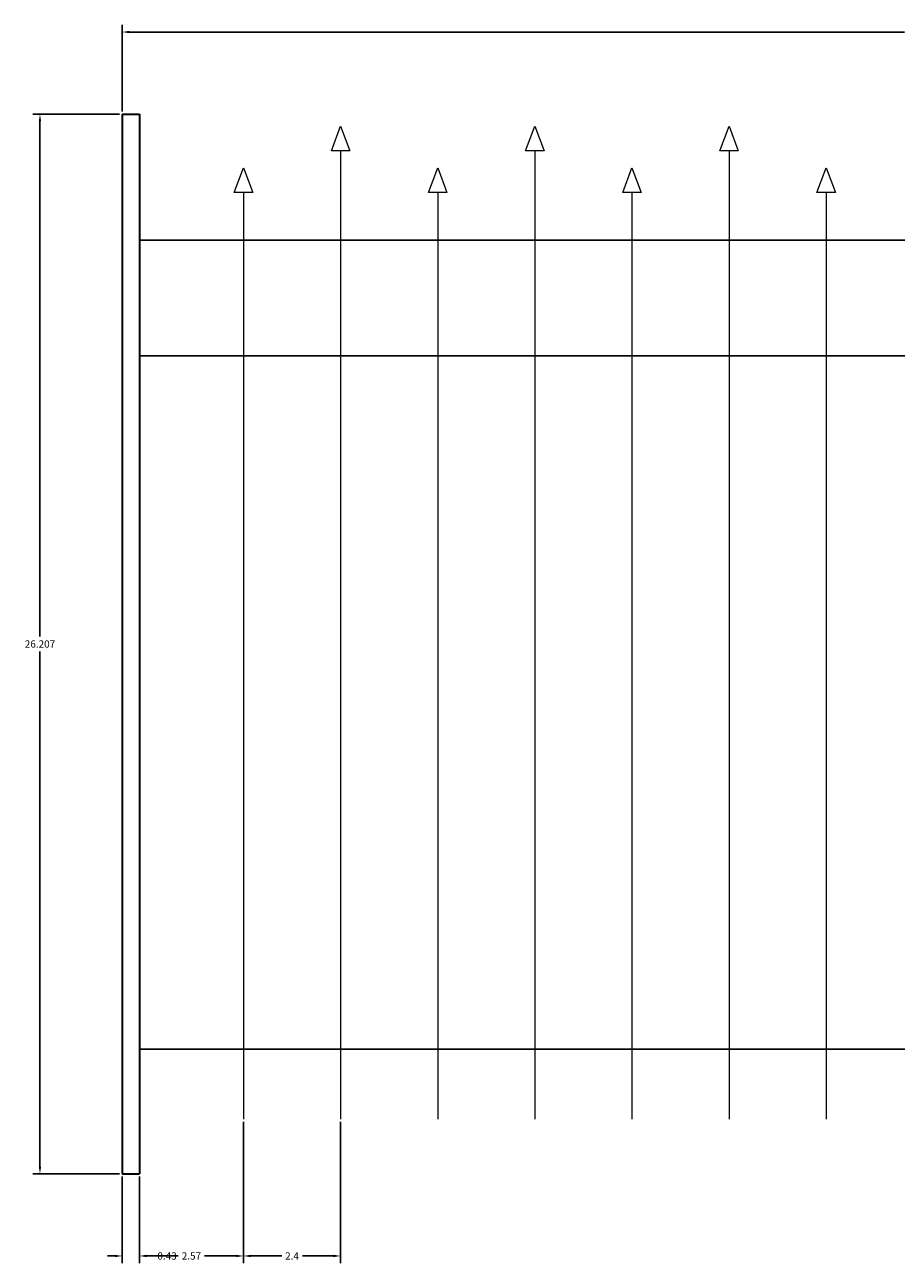
# Model space of a CAD drawing. Units: inches. Extents: x 756 to 915, y 488 to 695.
# Tile 17 of 25: x 768 to 789, y 664 to 694. Entities that reach past the tile are written whole.
import ezdxf

# ---------------------------------------------------------------- set-up
doc = ezdxf.new("R2010")
doc.units = ezdxf.units.IN
doc.header["$MEASUREMENT"] = 0
for name, color, linetype, lineweight in [('L-FENC-PCKT', 7, 'Continuous', 18), ('L-FENC-POST', 7, 'Continuous', 35), ('L-FENC-RAIL', 7, 'Continuous', 25), ('M-DIMS', 2, 'Continuous', 18)]:
    doc.layers.add(name, color=color, linetype=linetype, lineweight=lineweight)
doc.styles.get("Standard").update_dxf_attribs({"font": 'arial.ttf'})
doc.dimstyles.get("Standard").update_dxf_attribs({"dimtxt": 0.18, "dimasz": 0.18, "dimexe": 0.18, "dimexo": 0.0625, "dimgap": 0.09, "dimtad": 0, "dimtih": 1, "dimtoh": 1, "dimdec": 0, "dimzin": 0, "dimdsep": 46, "dimlunit": 3, "dimtxsty": 'Standard', "dimcen": 0.09, "dimadec": 0, "dimazin": 0, "dimtfac": 1, "dimtdec": 0, "dimtofl": 0, "dimtmove": 0, "dimatfit": 3, "dimfxl": 1, "dimtolj": 1, "dimtzin": 0, "dimarcsym": 0})

# ---------------------------------------------------------------- blocks, each defined once
blk = doc.blocks.new('PICKET-SPEAR-EXTENDED')
blk.add_line((0.228, 23.946), (0.228, 0))
blk.add_lwpolyline([(0.228, 23.946), (0, 23.946), (0.228, 24.558), (0.455, 23.946)], close=True)
blk = doc.blocks.new('FENCE-POST-LEFT')
for p, q in [((0, 26.207), (0, 0)), ((0, 26.207), (0.426, 26.207)), ((0.426, 26.207), (0.426, 0)), ((0.426, 26.207), (0.426, 0)), ((0, 0), (0.426, 0))]:
    blk.add_line(p, q)
blk = doc.blocks.new('PICKET-SPEAR-LOW')
blk.add_line((0.228, 22.916), (0.228, 0))
blk.add_lwpolyline([(0.228, 22.916), (0, 22.916), (0.228, 23.528), (0.455, 22.916)], close=True)
blk = doc.blocks.new('*D13')
at = {"layer": 'Defpoints', "color": 0, "transparency": 16777216}
for p in [(809.674, 693.983), (770.216, 691.953), (809.674, 691.953)]:
    blk.add_point(p, dxfattribs=at)
at = {"layer": 'M-DIMS', "color": 0, "lineweight": -2, "transparency": 16777216}
for p, q in [((770.216, 692.015), (770.216, 694.163)), ((809.674, 692.015), (809.674, 694.163)), ((770.396, 693.983), (789.551, 693.983)), ((809.494, 693.983), (790.338, 693.983))]:
    blk.add_line(p, q, dxfattribs=at)
at = {"layer": 'M-DIMS', "color": 0, "transparency": 16777216}
for points in [[(770.396, 694.013), (770.396, 693.953), (770.216, 693.983)], [(809.494, 694.013), (809.494, 693.953), (809.674, 693.983)]]:
    blk.add_solid(points, dxfattribs=at)
at = {"layer": 'M-DIMS', "color": 0, "transparency": 16777216, "insert": (789.945, 693.983), "char_height": 0.18, "attachment_point": 5}
blk.add_mtext('\\A1;39.46', dxfattribs=at)
blk = doc.blocks.new('*D14')
at = {"layer": 'Defpoints', "color": 0, "transparency": 16777216}
for p in [(768.186, 691.953), (770.216, 691.953), (770.216, 665.746)]:
    blk.add_point(p, dxfattribs=at)
at = {"layer": 'M-DIMS', "color": 0, "lineweight": -2, "transparency": 16777216}
for p, q in [((770.153, 691.953), (768.006, 691.953)), ((768.186, 691.773), (768.186, 679.031)), ((768.186, 665.926), (768.186, 678.668)), ((770.153, 665.746), (768.006, 665.746))]:
    blk.add_line(p, q, dxfattribs=at)
at = {"layer": 'M-DIMS', "color": 0, "transparency": 16777216}
for points in [[(768.156, 691.773), (768.216, 691.773), (768.186, 691.953)], [(768.156, 665.926), (768.216, 665.926), (768.186, 665.746)]]:
    blk.add_solid(points, dxfattribs=at)
at = {"layer": 'M-DIMS', "color": 0, "transparency": 16777216, "insert": (768.186, 678.849), "char_height": 0.18, "attachment_point": 5}
blk.add_mtext('\\A1;26.207', dxfattribs=at)
blk = doc.blocks.new('*D15')
at = {"layer": 'Defpoints', "color": 0, "transparency": 16777216}
for p in [(773.215, 667.096), (775.615, 667.096), (775.615, 663.716)]:
    blk.add_point(p, dxfattribs=at)
at = {"layer": 'M-DIMS', "color": 0, "lineweight": -2, "transparency": 16777216}
for p, q in [((773.215, 667.033), (773.215, 663.536)), ((775.615, 667.033), (775.615, 663.536)), ((773.395, 663.716), (774.16, 663.716)), ((775.435, 663.716), (774.67, 663.716))]:
    blk.add_line(p, q, dxfattribs=at)
at = {"layer": 'M-DIMS', "color": 0, "transparency": 16777216}
for points in [[(773.395, 663.746), (773.395, 663.686), (773.215, 663.716)], [(775.435, 663.746), (775.435, 663.686), (775.615, 663.716)]]:
    blk.add_solid(points, dxfattribs=at)
at = {"layer": 'M-DIMS', "color": 0, "transparency": 16777216, "insert": (774.415, 663.716), "char_height": 0.18, "attachment_point": 5}
blk.add_mtext('\\A1;2.4', dxfattribs=at)
blk = doc.blocks.new('*D16')
at = {"layer": 'Defpoints', "color": 0, "transparency": 16777216}
for p in [(773.215, 667.096), (770.642, 665.746), (773.215, 663.716)]:
    blk.add_point(p, dxfattribs=at)
at = {"layer": 'M-DIMS', "color": 0, "lineweight": -2, "transparency": 16777216}
for p, q in [((773.215, 667.033), (773.215, 663.536)), ((770.642, 665.684), (770.642, 663.536)), ((770.822, 663.716), (771.603, 663.716)), ((773.035, 663.716), (772.254, 663.716))]:
    blk.add_line(p, q, dxfattribs=at)
at = {"layer": 'M-DIMS', "color": 0, "transparency": 16777216}
for points in [[(770.822, 663.746), (770.822, 663.686), (770.642, 663.716)], [(773.035, 663.746), (773.035, 663.686), (773.215, 663.716)]]:
    blk.add_solid(points, dxfattribs=at)
at = {"layer": 'M-DIMS', "color": 0, "transparency": 16777216, "insert": (771.929, 663.716), "char_height": 0.18, "attachment_point": 5}
blk.add_mtext('\\A1;2.57', dxfattribs=at)
blk = doc.blocks.new('*D18')
at = {"layer": 'Defpoints', "color": 0, "transparency": 16777216}
for p in [(770.216, 665.746), (770.642, 665.746), (770.642, 663.716)]:
    blk.add_point(p, dxfattribs=at)
at = {"layer": 'M-DIMS', "color": 0, "lineweight": -2, "transparency": 16777216}
for p, q in [((770.216, 665.684), (770.216, 663.536)), ((770.642, 665.684), (770.642, 663.536)), ((770.036, 663.716), (769.856, 663.716)), ((770.822, 663.716), (771.002, 663.716))]:
    blk.add_line(p, q, dxfattribs=at)
at = {"layer": 'M-DIMS', "color": 0, "transparency": 16777216}
for points in [[(770.036, 663.746), (770.036, 663.686), (770.216, 663.716)], [(770.822, 663.746), (770.822, 663.686), (770.642, 663.716)]]:
    blk.add_solid(points, dxfattribs=at)
at = {"layer": 'M-DIMS', "color": 0, "transparency": 16777216, "insert": (771.326, 663.716), "char_height": 0.18, "attachment_point": 5}
blk.add_mtext('\\A1;0.43', dxfattribs=at)

msp = doc.modelspace()

# ---------------------------------------------------------------- linework, layer by layer
at = {"layer": 'L-FENC-RAIL'}
for p, q in [((770.6423, 688.8379), (809.2471, 688.8379)), ((770.6423, 685.9735), (809.2471, 685.9735)), ((770.6423, 668.8277), (809.2471, 668.8277))]:
    msp.add_line(p, q, dxfattribs=at)

# ---------------------------------------------------------------- block references
at = {"layer": 'L-FENC-PCKT'}
for name, p in [('PICKET-SPEAR-EXTENDED', (775.387, 667.096)), ('PICKET-SPEAR-EXTENDED', (780.1868, 667.096)), ('PICKET-SPEAR-EXTENDED', (784.9866, 667.096)), ('PICKET-SPEAR-LOW', (772.987, 667.096)), ('PICKET-SPEAR-LOW', (777.7868, 667.096)), ('PICKET-SPEAR-LOW', (782.5866, 667.096)), ('PICKET-SPEAR-LOW', (787.3865, 667.096))]:
    msp.add_blockref(name, p, dxfattribs=at)
at = {"layer": 'L-FENC-POST'}
msp.add_blockref('FENCE-POST-LEFT', (770.216, 665.746), dxfattribs=at)

# ---------------------------------------------------------------- dimensions: what is measured, and where the dimension line sits
at = {"layer": 'M-DIMS'}
for base, p1, p2, override, picture, middle in [((809.6738, 693.9829), (770.2156, 691.9529), (809.6738, 691.9529), {"dimdec": 2, "dimlfac": 1, "dimrnd": 0, "dimzin": 0, "dimdsep": 46, "dimlunit": 2}, '*D13', (789.9447, 693.9829)), ((773.2147, 663.7161), (770.6423, 665.7461), (773.2147, 667.0956), {"dimdec": 2, "dimlfac": 1, "dimrnd": 0, "dimzin": 0, "dimdsep": 46, "dimlunit": 2}, '*D16', (771.9285, 663.7161)), ((775.6147, 663.7161), (773.2147, 667.0956), (775.6147, 667.0956), {"dimdec": 1, "dimlfac": 1, "dimrnd": 0, "dimzin": 0, "dimdsep": 46, "dimlunit": 2}, '*D15', (774.4147, 663.7161)), ((770.6423, 663.7161), (770.2156, 665.7461), (770.6423, 665.7461), {"dimdec": 2, "dimlfac": 1, "dimrnd": 0, "dimzin": 0, "dimdsep": 46, "dimlunit": 2}, '*D18', (771.3261, 663.7161))]:
    dim = msp.add_linear_dim(base=base, p1=p1, p2=p2, dimstyle='Standard', override=override, dxfattribs=at)
    dim.commit()
    dim.dimension.update_dxf_attribs({"geometry": picture, "text_midpoint": middle})
dim = msp.add_linear_dim(base=(768.1856, 691.9529), p1=(770.2156, 665.7461), p2=(770.2156, 691.9529), angle=90, dimstyle='Standard', override={"dimdec": 3, "dimlfac": 1, "dimrnd": 0, "dimzin": 0, "dimdsep": 46, "dimlunit": 2}, dxfattribs=at)
dim.commit()
dim.dimension.update_dxf_attribs({"geometry": '*D14', "text_midpoint": (768.1856, 678.8495)})

doc.saveas('drawing.dxf')
